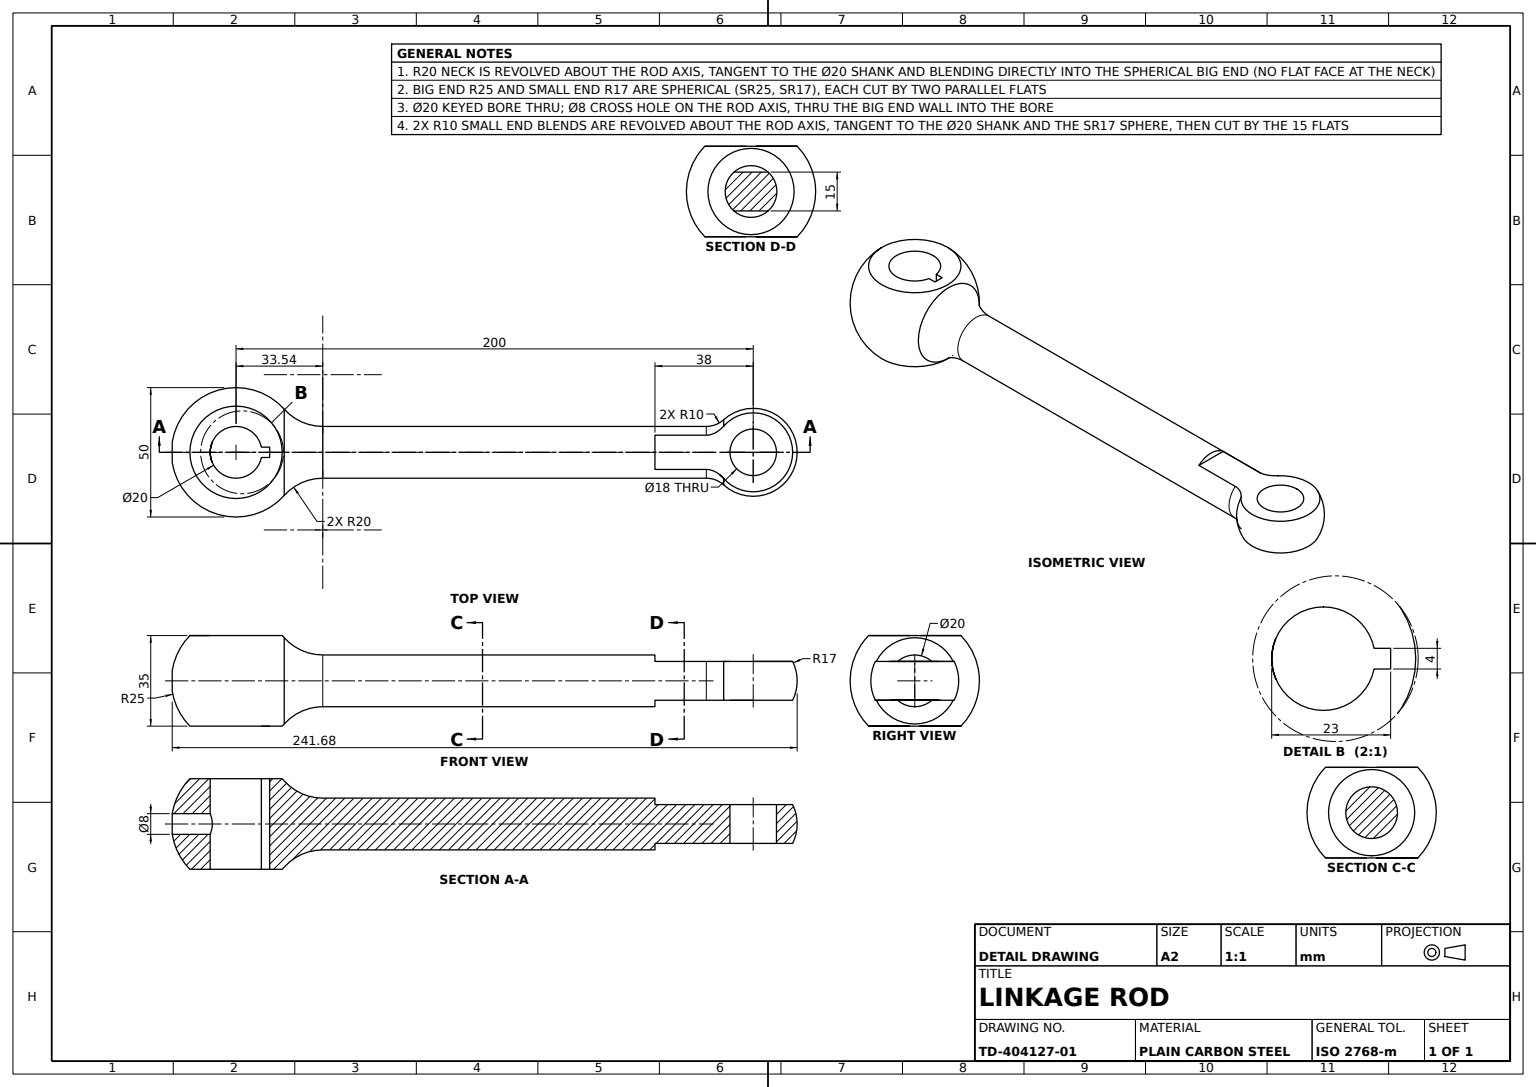
SolidWorks part; units mm, degrees
material "Plain Carbon Steel"
ref_plane "Front Plane" through (0, 0, 0) normal (0, 0, 1) x (1, 0, 0)
ref_plane "Top Plane" through (0, 0, 0) normal (0, 1, 0) x (1, 0, 0)
ref_plane "Right Plane" through (0, 0, 0) normal (1, 0, 0) x (0, 0, -1)
sketch "Rod Profile Sketch" plane through (0, 0, 0) normal (0, 0, 1) x (1, 0, 0)
  line L0 (-2.0871, 10) -> (161.2523, 10)
  line L1 (0, 0) -> (230.3752, 0) construction
  line L2 (-50, 0) -> (192, 0)
  arc A0 (161.2523, 10) -> (192, 0) centre (175, 0) cw
  arc A1 (-2.0871, 10) -> (-50, 0) centre (-25, 0) ccw
  dimension "D3" = 25
  dimension "D4" = 17
  dimension "D1" = 200
  dimension "D2" = 20
revolve "Rod Body Revolve" add sketch "Rod Profile Sketch" angle 360 about L1
ref_plane "Small End Flat Plane" through (0, 7.5, 0) normal (0, 1, 0) x (1, 0, 0)
sketch "Small End Flat Sketch" plane through (0, 7.5, 0) normal (0, 1, 0) x (1, 0, 0)
  line L0 (137.0022, 20.2694) -> (137.0022, -16.5212)
  line L1 (137.0022, -16.5212) -> (192.0022, -16.5212)
  line L2 (192.0022, -16.5212) -> (192.0022, 18.0085)
  line L3 (192.0022, 18.0085) -> (137.0022, 20.2694)
  dimension "D1" = 55
  dimension "D2" = 137.0022
  dimension "D3" = 16.5212
  dimension "D4" = 36.7906
  dimension "D5" = 34.5297
extrude "Small End Flat" cut sketch "Small End Flat Sketch" along normal blind 10
mirror "Small End Flat Mirror" about plane through (0, 0, 0) normal (0, 1, 0) of "Small End Flat"
ref_plane "Big End Flat Plane" through (0, 17.5, 0) normal (0, 1, 0) x (1, 0, 0)
sketch "Big End Flat Sketch" plane through (0, 17.5, 0) normal (0, 1, 0) x (1, 0, 0)
  line L1 (-68.4902, 27.7466) -> (18.4902, 27.7466)
  line L2 (-68.4902, 27.7466) -> (-68.4902, -27.7466)
  line L3 (-68.4902, -27.7466) -> (18.4902, -27.7466)
  line L4 (18.4902, 27.7466) -> (18.4902, -27.7466)
  line L5 (-68.4902, 27.7466) -> (18.4902, -27.7466) construction
  line L6 (-68.4902, -27.7466) -> (18.4902, 27.7466) construction
  point P0 (-25, 0)
  dimension "D1" = 25
  dimension "D2" = 86.9804
  dimension "D3" = 55.4933
extrude "Big End Flat" cut sketch "Big End Flat Sketch" along normal blind 10
mirror "Big End Flat Mirror" about plane through (0, 0, 0) normal (0, 1, 0) of "Big End Flat"
sketch "Keyed Bore Sketch" plane through (0, 17.5, 0) normal (0, 1, 0) x (1, 0, 0)
  line L1 (-15.202, 2) -> (-12, 2)
  line L3 (-15.202, -2) -> (-12, -2)
  line L4 (-12, 2) -> (-12, -2)
  line L5 (-18, 2) -> (-12, -2) construction
  line L6 (-18, -2) -> (-12, 2) construction
  arc A0 (-15.202, 2) -> (-15.202, -2) centre (-25, 0) ccw
  circle A1 centre (-25, 0) radius 17.8536 construction
  point P4 (-15, 0)
  dimension "D1" = 20
  dimension "D2" = 4
  dimension "D3" = 23
extrude "Keyed Bore Ø20" cut sketch "Keyed Bore Sketch" against normal blind 40
sketch "Small End Hole Sketch" plane through (0, 7.5, 0) normal (0, 1, 0) x (1, 0, 0)
  circle A0 centre (175, 0) radius 9
  arc A1 (161.2523, -6.6144) -> (161.2523, 6.6144) centre (175, 0) ccw construction
  dimension "D1" = 18
extrude "Small End Hole" cut sketch "Small End Hole Sketch" against normal blind 40
fillet "Fillet R20" radius 20 1 edges at (-2.0871, 0, 10)
fillet "Fillet R10" radius 10 2 edges at (161.2523, 0, 10) (161.2523, 0, -10)
ref_plane "Cross Hole Plane" through (-50, 0, 0) normal (1, 0, 0) x (0, 0, -1)
sketch "Cross Hole Sketch" plane through (-50, 0, 0) normal (1, 0, 0) x (0, 0, -1)
  circle A0 centre (0, 0) radius 4
  dimension "D1" = 8
extrude "Cross Hole Ø8" cut sketch "Cross Hole Sketch" along normal blind 20
